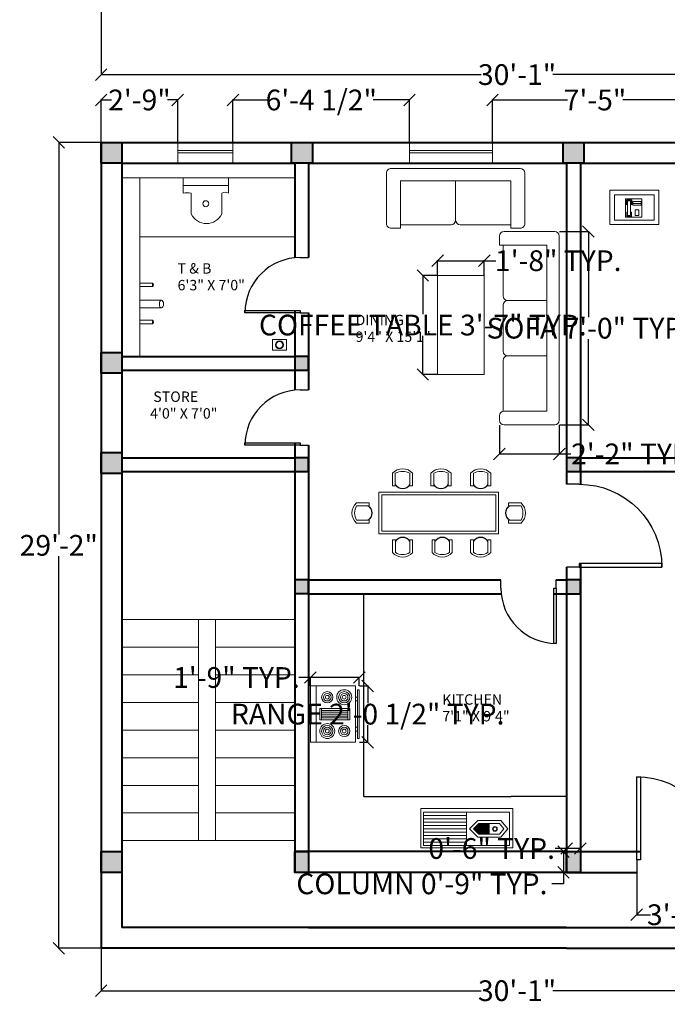
# Model space of a CAD drawing. Units: inches. Extents: x -19 to 1000, y -122 to 1144.
# Tile 4 of 8: x 529 to 810, y -115 to 313. Entities that reach past the tile are written whole.
import ezdxf

# ---------------------------------------------------------------- set-up
doc = ezdxf.new("R2010")
doc.units = ezdxf.units.IN
doc.header["$MEASUREMENT"] = 0
for name, color, linetype, lineweight in [('A-ANNO-DIMS', 191, 'Continuous', 18), ('A-AREA-IDEN', 1, 'Continuous', 18), ('A-COLS', 4, 'Continuous', 40), ('A-COLS-PATT', 220, 'Continuous', 13), ('A-EQPM', 120, 'Continuous', 18), ('A-FLOR-CASE', 254, 'Continuous', 25), ('A-FLOR-FIXT', 8, 'Continuous', 18), ('A-FLOR-STRS', 241, 'Continuous', 18), ('DOORS', 2, 'Continuous', 25), ('FURNITURE', 120, 'Continuous', 18), ('WALLS', 4, 'Continuous', 40), ('WINDOWS', 3, 'Continuous', 18)]:
    doc.layers.add(name, color=color, linetype=linetype, lineweight=lineweight)
doc.styles.get("Standard").update_dxf_attribs({"font": 'arial.ttf'})
doc.dimstyles.get("Standard").update_dxf_attribs({"dimtxt": 9, "dimasz": 5, "dimexe": 0.18, "dimexo": 0.0625, "dimgap": 0.09, "dimtad": 0, "dimtih": 1, "dimtoh": 1, "dimdec": 0, "dimzin": 0, "dimdsep": 46, "dimlunit": 3, "dimtxsty": 'Standard', "dimblk": 'OBLIQUE', "dimcen": 0.09, "dimadec": 0, "dimazin": 0, "dimtfac": 1, "dimtdec": 0, "dimtofl": 0, "dimtmove": 0, "dimatfit": 3, "dimfxl": 1, "dimtolj": 1, "dimtzin": 0, "dimarcsym": 0})

# ---------------------------------------------------------------- blocks, each defined once
blk = doc.blocks.new('Phone - Desk')
for p, q in [((-4.5, -5), (-4.5, 5)), ((-4.5, 5), (4.5, 5)), ((-4, 4.5), (-4, 2)), ((-4, 2), (-3.25, 2)), ((-3.75, 4.5), (-3.75, 2.25)), ((-1.25, 4.5), (-3.75, 4.5)), ((-3.75, 2.25), (-3.25, 2.25)), ((-3.25, 4), (-3.25, -4)), ((-3.25, 4), (-1.75, 4)), ((-1.75, -4), (-1.75, 4)), ((-1.75, 2.25), (-1.25, 2.25)), ((-1.75, 2), (-1, 2)), ((-1.25, 2.25), (-1.25, 4.5)), ((-1, 2), (-1, 4.5)), ((4, 3.5), (-0.5, 3.5)), ((-0.5, 3.5), (-0.5, 1.5)), ((-0.5, 2.5), (4, 2.5)), ((-0.5, 1.5), (4, 1.5)), ((4, 1.5), (4, 3.5)), ((4.5, 5), (4.5, -5)), ((4.5, -5), (-4.5, -5)), ((-3.75, -2.25), (-3.25, -2.25)), ((-3.75, -4.5), (-3.75, -2.25)), ((-1.25, -4.5), (-3.75, -4.5)), ((-3.25, -4), (-1.75, -4)), ((-1.75, -2.25), (-1.25, -2.25)), ((-1.25, -2.25), (-1.25, -4.5)), ((2.75, -1), (0.75, -1)), ((0.75, -1), (0.75, -4)), ((0.75, -4), (2.75, -4)), ((2.75, -4), (2.75, -1))]:
    blk.add_line(p, q)
blk = doc.blocks.new('Range-Oven - 30 in top')
for p, q in [((0, -3), (30, -3)), ((12, -6), (18, -6)), ((13, -20), (13, -6)), ((14, -6), (14, -20)), ((15, -20), (15, -6)), ((16, -6), (16, -20)), ((17, -20), (17, -6)), ((18, -20), (12, -20)), ((6, -24), (6, -25)), ((8, -25), (8, -24)), ((22, -25), (22, -24)), ((24, -24), (24, -25))]:
    blk.add_line(p, q)
for points in [[(0, -24), (0, 0), (30, 0), (30, -24)], [(12, -21), (12, -5), (18, -5), (18, -21)], [(2, -26), (2, -25), (28, -25), (28, -26)]]:
    blk.add_lwpolyline(points, close=True)
for centre, radius in [((6, -9), 4), ((6, -9), 3), ((6, -9), 2), ((6, -9), 1), ((24, -9), 3), ((24, -9), 2), ((24, -9), 1), ((6, -18), 3), ((24, -18), 4), ((24, -18), 3), ((6, -18), 2), ((6, -18), 1), ((24, -18), 2), ((24, -18), 1)]:
    blk.add_circle(centre, radius)
blk = doc.blocks.new('*U3')
for p, q in [((0, 0), (0, -6)), ((40, 0), (40, -6))]:
    blk.add_line(p, q)
blk.add_lwpolyline([(0, 0), (0, 40), (1.75, 40), (1.75, 0)], close=True)
blk.add_arc((0, 0), 40, 0, 90)
blk = doc.blocks.new('SOFA-THREE-SEAT')
for p, q in [((0, 78), (0, 82)), ((2, 84), (24, 84)), ((26, 82), (26, 2)), ((0, 78), (20.62, 78)), ((1.56, 78), (1.56, 56)), ((20.62, 78), (20.62, 6)), ((1.56, 52), (1.56, 32)), ((3.56, 54), (20.62, 54)), ((3.56, 54), (3.56, 54)), ((3.56, 30), (20.62, 30)), ((3.56, 30), (3.56, 30)), ((1.56, 28), (1.56, 6)), ((2, 6), (20.62, 6)), ((0, 2), (0, 4)), ((24, 0), (2, 0))]:
    blk.add_line(p, q)
for centre, start, end in [((2, 82), 90, 180), ((24, 82), 0, 90), ((3.56, 56), 180, 270), ((3.56, 52), 90, 180), ((3.56, 32), 180, 270), ((3.56, 28), 90, 180), ((2, 4), 90, 180), ((2, 2), 180, 270), ((24, 2), 270, 0)]:
    blk.add_arc(centre, 2, start, end)
blk = doc.blocks.new('LOVESEAT')
for p, q in [((6, 20.62), (54, 20.62)), ((6, 0), (6, 20.62)), ((30, 3.56), (30, 20.62)), ((54, 0), (54, 20.62)), ((6, 1.56), (28, 1.56)), ((30, 3.56), (30, 3.56)), ((32, 1.56), (54, 1.56))]:
    blk.add_line(p, q)
blk.add_lwpolyline([(6, 0), (2, 0, -0.414214), (0, 2), (0, 24, -0.414214), (2, 26), (58, 26, -0.414213), (60, 24), (60, 2, -0.414214), (58, 0), (54, 0)], format="xyb")
for centre, start, end in [((28, 3.56), 270, 0), ((32, 3.56), 180, 270)]:
    blk.add_arc(centre, 2, start, end)
blk = doc.blocks.new('TABLE-COFFEE')
blk.add_lwpolyline([(20.25, 0), (0, 0), (0, 43), (20.25, 43)], close=True)
blk = doc.blocks.new('TABLE-DINING')
for points in [[(51.97, 0), (0, 0), (0, 18.2), (51.97, 18.2)], [(50.72, 1.24), (1.24, 1.24), (1.24, 16.96), (50.72, 16.96)]]:
    blk.add_lwpolyline(points, close=True)
blk = doc.blocks.new('TABLE-BEDSIDE')
for points in [[(0, 0), (21.2, 0), (21.2, 14.94), (0, 14.94)], [(2, 2), (19.2, 2), (19.2, 12.94), (2, 12.94)]]:
    blk.add_lwpolyline(points, close=True)
blk = doc.blocks.new('CHAIR-DINING')
for p, q in [((0, 1.28), (0, 6.78)), ((1.24, 1.28), (1.24, 6.78)), ((7.52, 1.28), (7.52, 6.78)), ((8.77, 1.28), (8.77, 6.78)), ((0, 1.28), (1.24, 1.28)), ((7.52, 1.28), (8.77, 1.28))]:
    blk.add_line(p, q)
for centre, radius, start, end in [((4.38, 2.88), 5.87, 41.6504, 138.3496), ((4.38, 1.47), 6.17, 59.4137, 120.5863), ((4.38, 3.81), 3.65, 210.7965, 329.2035), ((4.38, 3.65), 3.65, 210.7965, 329.2035)]:
    blk.add_arc(centre, radius, start, end)
blk = doc.blocks.new('SINK-WITH-DRAINBOARD')
for p, q in [((19.91, 15.5), (1.26, 15.5)), ((19.91, 14.06), (1.26, 14.06)), ((19.91, 1.08), (19.91, 15.5)), ((19.91, 12.62), (1.26, 12.62)), ((19.91, 11.17), (1.26, 11.17)), ((19.91, 9.73), (1.26, 9.73)), ((24.75, 11.88), (21.21, 8.28)), ((25.28, 10.62), (22.97, 8.28)), ((23.36, 8.67), (29.71, 8.67)), ((23.74, 9.06), (29.71, 9.06)), ((24.12, 9.45), (29.71, 9.45)), ((24.51, 9.84), (29.71, 9.84)), ((24.75, 11.88), (34.73, 11.88)), ((24.89, 10.23), (29.71, 10.23)), ((25.28, 10.62), (34.14, 10.62)), ((25.28, 10.62), (29.71, 10.62)), ((29.71, 5.94), (29.71, 10.62)), ((34.14, 10.62), (36.12, 8.28)), ((34.73, 11.88), (37.76, 8.28)), ((19.91, 8.29), (1.26, 8.29)), ((19.91, 6.85), (1.26, 6.85)), ((19.91, 5.4), (1.26, 5.4)), ((24.75, 4.68), (21.21, 8.28)), ((25.28, 5.94), (22.97, 8.28)), ((22.97, 8.28), (29.71, 8.28)), ((23.36, 7.89), (29.71, 7.89)), ((23.74, 7.5), (29.71, 7.5)), ((24.12, 7.11), (29.71, 7.11)), ((24.51, 6.72), (29.71, 6.72)), ((24.75, 4.68), (34.73, 4.68)), ((24.89, 6.33), (29.71, 6.33)), ((25.28, 5.94), (34.14, 5.94)), ((34.14, 5.94), (36.12, 8.28)), ((34.73, 4.68), (37.76, 8.28)), ((19.91, 3.96), (1.26, 3.96)), ((19.91, 2.52), (1.26, 2.52))]:
    blk.add_line(p, q)
for points in [[(40, 0), (0, 0), (0, 17.1), (40, 17.1)], [(38.55, 1.08), (1.26, 1.08), (1.26, 15.5), (38.55, 15.5)]]:
    blk.add_lwpolyline(points, close=True)
for radius in [1.01, 0.803]:
    blk.add_circle((32.21, 8.28), radius)
blk = doc.blocks.new('WC-PLAN')
for p, q in [((0, 13.24), (0, 19.84)), ((0, 19.84), (19.57, 19.84)), ((19.57, 13.24), (19.57, 19.84)), ((0, 16.54), (19.57, 16.54)), ((3.44, 13.24), (3.44, 4.14)), ((16.7, 13.24), (16.7, 4.14))]:
    blk.add_line(p, q)
blk.add_circle((9.78, 8.6), 1.3)
for centre, radius, start, end in [((1.72, 2.24), 11.13, 81.1156, 98.8844), ((18.13, 10.18), 3.38, 64.9191, 115.0809), ((10.07, 7.39), 7.39, 206.0978, 333.9022)]:
    blk.add_arc(centre, radius, start, end)
blk = doc.blocks.new('FLOOR-DRAIN')
blk.add_lwpolyline([(6.19, 0), (0, 0), (0, 4.58), (6.19, 4.58)], close=True)
for radius in [1.73, 1.73, 1.73, 1.49]:
    blk.add_circle((3.09, 2.29), radius)
blk = doc.blocks.new('STAIR-RETURN-PLAN')
for p, q in [((75, 96), (0, 96)), ((33.21, 0), (33.21, 96)), ((40.68, 0), (40.68, 96)), ((33.21, 84), (0, 84)), ((75, 84), (40.68, 84)), ((33.21, 72), (0, 72)), ((75, 72), (40.68, 72)), ((33.21, 60), (0, 60)), ((75, 60), (40.68, 60)), ((33.21, 48), (0, 48)), ((75, 48), (40.68, 48)), ((33.21, 36), (0, 36)), ((75, 36), (40.68, 36)), ((33.21, 24), (0, 24)), ((75, 24), (40.68, 24)), ((33.21, 12), (0, 12)), ((75, 12), (40.68, 12)), ((75, 0), (0, 0))]:
    blk.add_line(p, q)
blk = doc.blocks.new('WIN-24-PLAN')
for p, q in [((0, 4.5), (0, 9)), ((0, 9), (0, 0)), ((24, 9), (24, 0)), ((0, 5.5), (24, 5.5)), ((0, 4.5), (24, 4.5))]:
    blk.add_line(p, q)
blk = doc.blocks.new('WIN-36-PLAN')
for p, q in [((0, 4.5), (0, 9)), ((0, 9), (0, 0)), ((36, 9), (36, 0)), ((0, 5.5), (36, 5.5)), ((0, 5.5), (36, 5.5)), ((0, 4.5), (36, 4.5))]:
    blk.add_line(p, q)
blk = doc.blocks.new('COLUMN-9X9')
blk.add_lwpolyline([(0, 9), (9, 9), (9, 0), (0, 0)], close=True)
blk = doc.blocks.new('COLUMN-6X6')
blk.add_lwpolyline([(6, 6), (0, 6), (0, 0), (6, 0)], close=True)
blk = doc.blocks.new('COLUMN-6X9')
blk.add_lwpolyline([(0, 9), (6, 9), (6, 0), (0, 0)], close=True)
blk = doc.blocks.new('_Oblique')
at = {"color": 0, "linetype": 'ByBlock', "lineweight": -2}
blk.add_line((-0.5, -0.5), (0.5, 0.5), dxfattribs=at)
blk = doc.blocks.new('*D37')
at = {"layer": 'A-ANNO-DIMS', "color": 0, "lineweight": -2, "transparency": 16777216}
for p, q in [((766.28, -48.29), (764.81, -48.29)), ((764.99, -48.29), (764.99, -57.29)), ((766.28, -57.29), (764.81, -57.29)), ((764.99, -57.29), (764.99, -62.29)), ((764.99, -62.29), (759.99, -62.29))]:
    blk.add_line(p, q, dxfattribs=at)
at = {"layer": 'Defpoints', "color": 0, "transparency": 16777216}
for p in [(766.34, -48.29), (764.99, -57.29), (766.34, -57.29)]:
    blk.add_point(p, dxfattribs=at)
at = {"layer": 'A-ANNO-DIMS', "color": 0, "lineweight": -2, "transparency": 16777216, "xscale": 5, "yscale": 5, "zscale": 5}
for p, rotation in [((764.99, -48.29), 90), ((764.99, -57.29), 270)]:
    blk.add_blockref('_Oblique', p, dxfattribs=dict(at, rotation=rotation))
at = {"layer": 'A-ANNO-DIMS', "color": 0, "transparency": 16777216, "insert": (703.54, -62.29), "char_height": 9, "attachment_point": 5}
blk.add_mtext('\\A1;COLUMN 0\'-9" TYP.', dxfattribs=at)
blk = doc.blocks.new('*D38')
at = {"layer": 'A-ANNO-DIMS', "color": 0, "lineweight": -2, "transparency": 16777216}
for p, q in [((766.34, -46.94), (761.34, -46.94)), ((766.34, -48.23), (766.34, -46.76)), ((772.34, -46.94), (766.34, -46.94)), ((772.34, -48.23), (772.34, -46.76))]:
    blk.add_line(p, q, dxfattribs=at)
at = {"layer": 'Defpoints', "color": 0, "transparency": 16777216}
for p in [(766.34, -46.94), (766.34, -48.29), (772.34, -48.29)]:
    blk.add_point(p, dxfattribs=at)
at = {"layer": 'A-ANNO-DIMS', "color": 0, "lineweight": -2, "transparency": 16777216, "xscale": 5, "yscale": 5, "zscale": 5, "rotation": 180}
blk.add_blockref('_Oblique', (766.34, -46.94), dxfattribs=at)
at = {"layer": 'A-ANNO-DIMS', "color": 0, "lineweight": -2, "transparency": 16777216, "xscale": 5, "yscale": 5, "zscale": 5}
blk.add_blockref('_Oblique', (772.34, -46.94), dxfattribs=at)
at = {"layer": 'A-ANNO-DIMS', "color": 0, "transparency": 16777216, "insert": (733.82, -46.94), "char_height": 9, "attachment_point": 5}
blk.add_mtext('\\A1;0\'-6" TYP.', dxfattribs=at)
blk = doc.blocks.new('*D51')
at = {"layer": 'A-ANNO-DIMS', "color": 0, "lineweight": -2, "transparency": 16777216}
for p, q in [((676.41, 23.65), (680.2, 23.65)), ((680.02, 23.65), (680.02, 16.16)), ((680.02, -0.82), (680.02, 6.67)), ((676.41, -0.82), (680.2, -0.82))]:
    blk.add_line(p, q, dxfattribs=at)
at = {"layer": 'Defpoints', "color": 0, "transparency": 16777216}
for p in [(676.35, 23.65), (680.02, 23.65), (676.35, -0.82)]:
    blk.add_point(p, dxfattribs=at)
at = {"layer": 'A-ANNO-DIMS', "color": 0, "lineweight": -2, "transparency": 16777216, "xscale": 5, "yscale": 5, "zscale": 5}
for p, rotation in [((680.02, 23.65), 90), ((680.02, -0.82), 270)]:
    blk.add_blockref('_Oblique', p, dxfattribs=dict(at, rotation=rotation))
at = {"layer": 'A-ANNO-DIMS', "color": 0, "transparency": 16777216, "insert": (680.02, 11.41), "char_height": 9, "attachment_point": 5}
blk.add_mtext('\\A1;RANGE 2\'-0 1/2" TYP.', dxfattribs=at)
blk = doc.blocks.new('*D52')
at = {"layer": 'A-ANNO-DIMS', "color": 0, "lineweight": -2, "transparency": 16777216}
for p, q in [((655.14, 27.32), (650.14, 27.32)), ((655.14, 23.71), (655.14, 27.5)), ((676.35, 27.32), (655.14, 27.32)), ((676.35, 23.71), (676.35, 27.5))]:
    blk.add_line(p, q, dxfattribs=at)
at = {"layer": 'Defpoints', "color": 0, "transparency": 16777216}
for p in [(655.14, 27.32), (655.14, 23.65), (676.35, 23.65)]:
    blk.add_point(p, dxfattribs=at)
at = {"layer": 'A-ANNO-DIMS', "color": 0, "lineweight": -2, "transparency": 16777216, "xscale": 5, "yscale": 5, "zscale": 5, "rotation": 180}
blk.add_blockref('_Oblique', (655.14, 27.32), dxfattribs=at)
at = {"layer": 'A-ANNO-DIMS', "color": 0, "lineweight": -2, "transparency": 16777216, "xscale": 5, "yscale": 5, "zscale": 5}
blk.add_blockref('_Oblique', (676.35, 27.32), dxfattribs=at)
at = {"layer": 'A-ANNO-DIMS', "color": 0, "transparency": 16777216, "insert": (623.05, 27.32), "char_height": 9, "attachment_point": 5}
blk.add_mtext('\\A1;1\'-9" TYP.', dxfattribs=at)
blk = doc.blocks.new('*D53')
at = {"layer": 'A-ANNO-DIMS', "color": 0, "lineweight": -2, "transparency": 16777216}
for p, q in [((763.25, 221.01), (775.96, 221.01)), ((775.78, 221.01), (775.78, 183.75)), ((775.78, 137.01), (775.78, 174.26)), ((763.25, 137.01), (775.96, 137.01))]:
    blk.add_line(p, q, dxfattribs=at)
at = {"layer": 'Defpoints', "color": 0, "transparency": 16777216}
for p in [(763.18, 221.01), (775.78, 221.01), (763.18, 137.01)]:
    blk.add_point(p, dxfattribs=at)
at = {"layer": 'A-ANNO-DIMS', "color": 0, "lineweight": -2, "transparency": 16777216, "xscale": 5, "yscale": 5, "zscale": 5}
for p, rotation in [((775.78, 221.01), 90), ((775.78, 137.01), 270)]:
    blk.add_blockref('_Oblique', p, dxfattribs=dict(at, rotation=rotation))
at = {"layer": 'A-ANNO-DIMS', "color": 0, "transparency": 16777216, "insert": (775.78, 179.01), "char_height": 9, "attachment_point": 5}
blk.add_mtext('\\A1;SOFA 7\'-0" TYP.', dxfattribs=at)
blk = doc.blocks.new('*D54')
at = {"layer": 'A-ANNO-DIMS', "color": 0, "lineweight": -2, "transparency": 16777216}
for p, q in [((737.18, 136.94), (737.18, 124.23)), ((763.18, 136.94), (763.18, 124.23)), ((737.18, 124.41), (763.18, 124.41)), ((763.18, 124.41), (768.18, 124.41))]:
    blk.add_line(p, q, dxfattribs=at)
at = {"layer": 'Defpoints', "color": 0, "transparency": 16777216}
for p in [(737.18, 137.01), (763.18, 137.01), (763.18, 124.41)]:
    blk.add_point(p, dxfattribs=at)
at = {"layer": 'A-ANNO-DIMS', "color": 0, "lineweight": -2, "transparency": 16777216, "xscale": 5, "yscale": 5, "zscale": 5, "rotation": 180}
blk.add_blockref('_Oblique', (737.18, 124.41), dxfattribs=at)
at = {"layer": 'A-ANNO-DIMS', "color": 0, "lineweight": -2, "transparency": 16777216, "xscale": 5, "yscale": 5, "zscale": 5}
blk.add_blockref('_Oblique', (763.18, 124.41), dxfattribs=at)
at = {"layer": 'A-ANNO-DIMS', "color": 0, "transparency": 16777216, "insert": (795.78, 124.41), "char_height": 9, "attachment_point": 5}
blk.add_mtext('\\A1;2\'-2" TYP.', dxfattribs=at)
blk = doc.blocks.new('*D57')
at = {"layer": 'A-ANNO-DIMS', "color": 0, "lineweight": -2, "transparency": 16777216}
for p, q in [((710.31, 201.87), (703.74, 201.87)), ((703.92, 201.87), (703.92, 185.12)), ((703.92, 158.87), (703.92, 175.62)), ((710.31, 158.87), (703.74, 158.87))]:
    blk.add_line(p, q, dxfattribs=at)
at = {"layer": 'Defpoints', "color": 0, "transparency": 16777216}
for p in [(703.92, 201.87), (710.37, 201.87), (710.37, 158.87)]:
    blk.add_point(p, dxfattribs=at)
at = {"layer": 'A-ANNO-DIMS', "color": 0, "lineweight": -2, "transparency": 16777216, "xscale": 5, "yscale": 5, "zscale": 5}
for p, rotation in [((703.92, 201.87), 90), ((703.92, 158.87), 270)]:
    blk.add_blockref('_Oblique', p, dxfattribs=dict(at, rotation=rotation))
at = {"layer": 'A-ANNO-DIMS', "color": 0, "transparency": 16777216, "insert": (703.92, 180.37), "char_height": 9, "attachment_point": 5}
blk.add_mtext('\\A1;COFFEE TABLE 3\'-7" TYP.', dxfattribs=at)
blk = doc.blocks.new('*D58')
at = {"layer": 'A-ANNO-DIMS', "color": 0, "lineweight": -2, "transparency": 16777216}
for p, q in [((710.37, 201.93), (710.37, 208.5)), ((710.37, 208.32), (730.62, 208.32)), ((730.62, 201.93), (730.62, 208.5)), ((730.62, 208.32), (735.62, 208.32))]:
    blk.add_line(p, q, dxfattribs=at)
at = {"layer": 'Defpoints', "color": 0, "transparency": 16777216}
for p in [(730.62, 208.32), (710.37, 201.87), (730.62, 201.87)]:
    blk.add_point(p, dxfattribs=at)
at = {"layer": 'A-ANNO-DIMS', "color": 0, "lineweight": -2, "transparency": 16777216, "xscale": 5, "yscale": 5, "zscale": 5, "rotation": 180}
blk.add_blockref('_Oblique', (710.37, 208.32), dxfattribs=at)
at = {"layer": 'A-ANNO-DIMS', "color": 0, "lineweight": -2, "transparency": 16777216, "xscale": 5, "yscale": 5, "zscale": 5}
blk.add_blockref('_Oblique', (730.62, 208.32), dxfattribs=at)
at = {"layer": 'A-ANNO-DIMS', "color": 0, "transparency": 16777216, "insert": (762.72, 208.32), "char_height": 9, "attachment_point": 5}
blk.add_mtext('\\A1;1\'-8" TYP.', dxfattribs=at)
blk = doc.blocks.new('*D103')
at = {"layer": 'A-ANNO-DIMS', "color": 0, "lineweight": -2, "transparency": 16777216}
for p, q in [((564.34, -90.36), (564.34, -108.87)), ((925.34, -90.36), (925.34, -108.87)), ((564.34, -108.69), (729.3, -108.69)), ((925.34, -108.69), (760.39, -108.69))]:
    blk.add_line(p, q, dxfattribs=at)
at = {"layer": 'Defpoints', "color": 0, "transparency": 16777216}
for p in [(564.34, -90.29), (925.34, -90.29), (925.34, -108.69)]:
    blk.add_point(p, dxfattribs=at)
at = {"layer": 'A-ANNO-DIMS', "color": 0, "lineweight": -2, "transparency": 16777216, "xscale": 5, "yscale": 5, "zscale": 5, "rotation": 180}
blk.add_blockref('_Oblique', (564.34, -108.69), dxfattribs=at)
at = {"layer": 'A-ANNO-DIMS', "color": 0, "lineweight": -2, "transparency": 16777216, "xscale": 5, "yscale": 5, "zscale": 5}
blk.add_blockref('_Oblique', (925.34, -108.69), dxfattribs=at)
at = {"layer": 'A-ANNO-DIMS', "color": 0, "transparency": 16777216, "insert": (744.84, -108.69), "char_height": 9, "attachment_point": 5}
blk.add_mtext('\\A1;30\'-1"', dxfattribs=at)
blk = doc.blocks.new('*D104')
at = {"layer": 'A-ANNO-DIMS', "color": 0, "lineweight": -2, "transparency": 16777216}
for p, q in [((564.28, 259.71), (545.76, 259.71)), ((545.94, 259.71), (545.94, 89.39)), ((545.94, -90.29), (545.94, 80.02)), ((564.28, -90.29), (545.76, -90.29))]:
    blk.add_line(p, q, dxfattribs=at)
at = {"layer": 'Defpoints', "color": 0, "transparency": 16777216}
for p in [(545.94, 259.71), (564.34, 259.71), (564.34, -90.29)]:
    blk.add_point(p, dxfattribs=at)
at = {"layer": 'A-ANNO-DIMS', "color": 0, "lineweight": -2, "transparency": 16777216, "xscale": 5, "yscale": 5, "zscale": 5}
for p, rotation in [((545.94, 259.71), 90), ((545.94, -90.29), 270)]:
    blk.add_blockref('_Oblique', p, dxfattribs=dict(at, rotation=rotation))
at = {"layer": 'A-ANNO-DIMS', "color": 0, "transparency": 16777216, "insert": (545.94, 84.71), "char_height": 9, "attachment_point": 5}
blk.add_mtext('\\A1;29\'-2"', dxfattribs=at)
blk = doc.blocks.new('*D105')
at = {"layer": 'A-ANNO-DIMS', "color": 0, "lineweight": -2, "transparency": 16777216}
for p, q in [((564.34, 259.77), (564.34, 278.29)), ((564.34, 278.11), (568.82, 278.11)), ((597.55, 278.11), (593.08, 278.11)), ((597.55, 259.77), (597.55, 278.29))]:
    blk.add_line(p, q, dxfattribs=at)
at = {"layer": 'Defpoints', "color": 0, "transparency": 16777216}
for p in [(597.55, 278.11), (564.34, 259.71), (597.55, 259.71)]:
    blk.add_point(p, dxfattribs=at)
at = {"layer": 'A-ANNO-DIMS', "color": 0, "lineweight": -2, "transparency": 16777216, "xscale": 5, "yscale": 5, "zscale": 5, "rotation": 180}
blk.add_blockref('_Oblique', (564.34, 278.11), dxfattribs=at)
at = {"layer": 'A-ANNO-DIMS', "color": 0, "lineweight": -2, "transparency": 16777216, "xscale": 5, "yscale": 5, "zscale": 5}
blk.add_blockref('_Oblique', (597.55, 278.11), dxfattribs=at)
at = {"layer": 'A-ANNO-DIMS', "color": 0, "transparency": 16777216, "insert": (580.95, 278.11), "char_height": 9, "attachment_point": 5}
blk.add_mtext('\\A1;2\'-9"', dxfattribs=at)
blk = doc.blocks.new('*D106')
at = {"layer": 'A-ANNO-DIMS', "color": 0, "lineweight": -2, "transparency": 16777216}
for p, q in [((621.55, 259.77), (621.55, 278.29)), ((621.55, 278.11), (637.3, 278.11)), ((698.18, 278.11), (682.43, 278.11)), ((698.18, 259.77), (698.18, 278.29))]:
    blk.add_line(p, q, dxfattribs=at)
at = {"layer": 'Defpoints', "color": 0, "transparency": 16777216}
for p in [(698.18, 278.11), (621.55, 259.71), (698.18, 259.71)]:
    blk.add_point(p, dxfattribs=at)
at = {"layer": 'A-ANNO-DIMS', "color": 0, "lineweight": -2, "transparency": 16777216, "xscale": 5, "yscale": 5, "zscale": 5, "rotation": 180}
blk.add_blockref('_Oblique', (621.55, 278.11), dxfattribs=at)
at = {"layer": 'A-ANNO-DIMS', "color": 0, "lineweight": -2, "transparency": 16777216, "xscale": 5, "yscale": 5, "zscale": 5}
blk.add_blockref('_Oblique', (698.18, 278.11), dxfattribs=at)
at = {"layer": 'A-ANNO-DIMS', "color": 0, "transparency": 16777216, "insert": (659.87, 278.11), "char_height": 9, "attachment_point": 5}
blk.add_mtext('\\A1;6\'-4 1/2"', dxfattribs=at)
blk = doc.blocks.new('*D107')
at = {"layer": 'A-ANNO-DIMS', "color": 0, "lineweight": -2, "transparency": 16777216}
for p, q in [((734.18, 259.77), (734.18, 278.29)), ((734.18, 278.11), (766.67, 278.11)), ((823.18, 278.11), (790.7, 278.11)), ((823.18, 259.77), (823.18, 278.29))]:
    blk.add_line(p, q, dxfattribs=at)
at = {"layer": 'Defpoints', "color": 0, "transparency": 16777216}
for p in [(823.18, 278.11), (734.18, 259.71), (823.18, 259.71)]:
    blk.add_point(p, dxfattribs=at)
at = {"layer": 'A-ANNO-DIMS', "color": 0, "lineweight": -2, "transparency": 16777216, "xscale": 5, "yscale": 5, "zscale": 5, "rotation": 180}
blk.add_blockref('_Oblique', (734.18, 278.11), dxfattribs=at)
at = {"layer": 'A-ANNO-DIMS', "color": 0, "lineweight": -2, "transparency": 16777216, "xscale": 5, "yscale": 5, "zscale": 5}
blk.add_blockref('_Oblique', (823.18, 278.11), dxfattribs=at)
at = {"layer": 'A-ANNO-DIMS', "color": 0, "transparency": 16777216, "insert": (778.68, 278.11), "char_height": 9, "attachment_point": 5}
blk.add_mtext('\\A1;7\'-5"', dxfattribs=at)
blk = doc.blocks.new('*D109')
at = {"layer": 'A-ANNO-DIMS', "color": 0, "lineweight": -2, "transparency": 16777216}
for p, q in [((796.78, -57.36), (796.78, -75.87)), ((832.78, -57.36), (832.78, -75.87)), ((796.78, -75.69), (802.73, -75.69)), ((832.78, -75.69), (826.83, -75.69))]:
    blk.add_line(p, q, dxfattribs=at)
at = {"layer": 'Defpoints', "color": 0, "transparency": 16777216}
for p in [(796.78, -57.29), (832.78, -57.29), (796.78, -75.69)]:
    blk.add_point(p, dxfattribs=at)
at = {"layer": 'A-ANNO-DIMS', "color": 0, "lineweight": -2, "transparency": 16777216, "xscale": 5, "yscale": 5, "zscale": 5, "rotation": 180}
blk.add_blockref('_Oblique', (796.78, -75.69), dxfattribs=at)
at = {"layer": 'A-ANNO-DIMS', "color": 0, "lineweight": -2, "transparency": 16777216, "xscale": 5, "yscale": 5, "zscale": 5}
blk.add_blockref('_Oblique', (832.78, -75.69), dxfattribs=at)
at = {"layer": 'A-ANNO-DIMS', "color": 0, "transparency": 16777216, "insert": (814.78, -75.69), "char_height": 9, "attachment_point": 5}
blk.add_mtext('\\A1;3\'-0"', dxfattribs=at)
blk = doc.blocks.new('*D129')
at = {"layer": 'A-ANNO-DIMS', "color": 0, "lineweight": -2, "transparency": 16777216}
for p, q in [((564.34, 328.07), (564.34, 288.95)), ((925.34, 328.07), (925.34, 288.95)), ((564.34, 289.13), (729.3, 289.13)), ((925.34, 289.13), (760.39, 289.13))]:
    blk.add_line(p, q, dxfattribs=at)
at = {"layer": 'Defpoints', "color": 0, "transparency": 16777216}
for p in [(564.34, 328.13), (925.34, 328.13), (925.34, 289.13)]:
    blk.add_point(p, dxfattribs=at)
at = {"layer": 'A-ANNO-DIMS', "color": 0, "lineweight": -2, "transparency": 16777216, "xscale": 5, "yscale": 5, "zscale": 5, "rotation": 180}
blk.add_blockref('_Oblique', (564.34, 289.13), dxfattribs=at)
at = {"layer": 'A-ANNO-DIMS', "color": 0, "lineweight": -2, "transparency": 16777216, "xscale": 5, "yscale": 5, "zscale": 5}
blk.add_blockref('_Oblique', (925.34, 289.13), dxfattribs=at)
at = {"layer": 'A-ANNO-DIMS', "color": 0, "transparency": 16777216, "insert": (744.84, 289.13), "char_height": 9, "attachment_point": 5}
blk.add_mtext('\\A1;30\'-1"', dxfattribs=at)

msp = doc.modelspace()

# ---------------------------------------------------------------- hatches: boundary and pattern name
at = {"layer": 'A-COLS-PATT'}
h = msp.add_hatch(color=256, dxfattribs=at)
h.dxf.hatch_style = 1
h.paths.add_polyline_path([(573.34, 259.71), (564.34, 259.71), (564.34, 250.71), (573.34, 250.71)])
h.paths.add_polyline_path([(656.01, 259.71), (647.01, 259.71), (647.01, 250.71), (656.01, 250.71)])
h.paths.add_polyline_path([(773.81, 259.71), (764.81, 259.71), (764.81, 250.71), (773.81, 250.71)])
h.paths.add_polyline_path([(925.34, 259.71), (916.34, 259.71), (916.34, 250.71), (925.34, 250.71)])
h = msp.add_hatch(color=256, dxfattribs=at)
h.dxf.hatch_style = 1
h.paths.add_polyline_path([(573.34, 168.48), (564.34, 168.48), (564.34, 159.48), (573.34, 159.48)])
h.paths.add_polyline_path([(654.34, 166.71), (648.34, 166.71), (648.34, 160.71), (654.34, 160.71)])
h.paths.add_polyline_path([(573.34, 124.97), (564.34, 124.97), (564.34, 115.97), (573.34, 115.97)])
h.paths.add_polyline_path([(654.34, 122.71), (648.34, 122.71), (648.34, 116.71), (654.34, 116.71)])
h.paths.add_polyline_path([(654.34, 69.8), (648.34, 69.8), (648.34, 63.8), (654.34, 63.8)])
h.paths.add_polyline_path([(772.34, 69.71), (766.34, 69.71), (766.34, 63.71), (772.34, 63.71)])
h.paths.add_polyline_path([(772.34, 122.71), (766.34, 122.71), (766.34, 116.71), (772.34, 116.71)])
h.paths.add_polyline_path([(925.34, 124.12), (916.34, 124.12), (916.34, 115.12), (925.34, 115.12)])
h.paths.add_polyline_path([(925.34, -48.29), (916.34, -48.29), (916.34, -57.29), (925.34, -57.29)])
h.paths.add_polyline_path([(772.34, -48.29), (766.34, -48.29), (766.34, -57.29), (772.34, -57.29)])
h.paths.add_polyline_path([(654.34, -48.29), (648.34, -48.29), (648.34, -57.29), (654.34, -57.29)])
h.paths.add_polyline_path([(573.34, -48.29), (564.34, -48.29), (564.34, -57.29), (573.34, -57.29)])

# ---------------------------------------------------------------- linework, layer by layer
at = {"layer": 'A-FLOR-CASE'}
for p, q in [((678.34, -24.29), (678.34, 63.71)), ((678.34, -24.29), (742.34, -24.29)), ((766.34, -24.29), (742.34, -24.29))]:
    msp.add_line(p, q, dxfattribs=at)
at = {"layer": 'A-FLOR-FIXT'}
for p, q in [((573.34, 244.3), (648.34, 244.3)), ((581.18, 166.71), (581.18, 244.3)), ((581.18, 218.69), (648.34, 218.69)), ((581.18, 198.59), (586.55, 198.59)), ((581.18, 197.08), (586.55, 197.08)), ((586.55, 198.59), (586.55, 197.08)), ((581.18, 191.12), (590.5, 191.12)), ((581.18, 187.85), (590.5, 187.85)), ((581.18, 182.45), (586.55, 182.45)), ((581.18, 180.94), (586.55, 180.94)), ((586.55, 182.45), (586.55, 180.94))]:
    msp.add_line(p, q, dxfattribs=at)
for centre in [(586.32, 197.83), (586.32, 181.69)]:
    msp.add_arc(centre, 0.786, 286.4895, 73.5105, dxfattribs=at)
msp.add_ellipse((590.5, 189.48), major_axis=(0, 1.63), ratio=0.555125, dxfattribs=at)
at = {"layer": 'WALLS'}
for p, q in [((564.34, 259.71), (564.34, -90.29)), ((564.34, 259.71), (925.34, 259.71)), ((573.34, 259.71), (573.34, -48.29)), ((573.34, 250.71), (648.34, 250.71)), ((648.34, 250.71), (648.34, 209.57)), ((654.34, 250.71), (654.34, 209.69)), ((654.34, 250.71), (766.34, 250.71)), ((766.34, 250.71), (766.34, 111.24)), ((772.34, 250.71), (772.34, 111.24)), ((772.34, 250.71), (916.34, 250.71)), ((648.34, 186.74), (648.34, 152.09)), ((654.34, 185.69), (654.34, 152.21)), ((573.34, 166.71), (648.34, 166.71)), ((573.34, 160.71), (648.34, 160.71)), ((648.34, 129.26), (648.34, -57.29)), ((654.34, 128.21), (654.34, -57.29)), ((573.34, 122.71), (648.34, 122.71)), ((772.34, 122.71), (916.34, 122.71)), ((573.34, 116.71), (648.34, 116.71)), ((772.34, 116.71), (916.34, 116.71)), ((766.34, 75.24), (766.34, -57.29)), ((772.34, 76.82), (772.34, -57.29)), ((654.34, 69.71), (737.83, 69.71)), ((761.83, 69.71), (766.34, 69.71)), ((654.34, 63.71), (737.95, 63.71)), ((760.78, 63.71), (766.34, 63.71)), ((766.34, -48.29), (648.34, -48.29)), ((766.34, -48.29), (798.35, -48.29)), ((573.34, -57.29), (573.34, -81.29)), ((766.34, -57.29), (648.34, -57.29)), ((766.34, -57.29), (796.78, -57.29)), ((766.34, -81.29), (573.34, -81.29)), ((654.34, -81.29), (916.34, -81.29)), ((766.34, -81.29), (654.34, -81.29)), ((654.34, -90.29), (564.34, -90.29)), ((766.34, -90.29), (654.34, -90.29)), ((766.34, -90.29), (925.34, -90.29))]:
    msp.add_line(p, q, dxfattribs=at)
msp.add_lwpolyline([(564.34, -57.29), (564.34, -48.29)], dxfattribs=at)

# ---------------------------------------------------------------- block references
at = {"layer": 'A-COLS'}
for p in [(564.34, 250.71), (647.01, 250.71), (764.81, 250.71), (564.34, 159.48), (564.34, 115.97), (564.34, -57.3)]:
    msp.add_blockref('COLUMN-9X9', p, dxfattribs=at)
for name, p, rotation in [('COLUMN-6X6', (648.34, 166.71), 270.0000000000003), ('COLUMN-6X6', (648.34, 122.71), 270.0000000000003), ('COLUMN-6X6', (766.34, 122.71), 270.0000000000013), ('COLUMN-6X6', (766.34, 122.71), 270.0000000000013), ('COLUMN-6X6', (648.34, 69.8), 270.0000000000003), ('COLUMN-6X6', (648.34, 69.8), 270.0000000000003), ('COLUMN-6X6', (766.34, 69.71), 270.0000000000013), ('COLUMN-6X9', (654.34, -48.29), 180), ('COLUMN-6X9', (772.34, -48.29), 180)]:
    msp.add_blockref(name, p, dxfattribs=dict(at, rotation=rotation))
at = {"layer": 'A-EQPM', "xscale": 0.8015722193121366, "yscale": 0.8015722193121366, "zscale": 0.8015722193121366}
msp.add_blockref('Phone - Desk', (795.45, 231.16), dxfattribs=at)
at = {"layer": 'A-EQPM', "xscale": 0.8155908971350484, "yscale": 0.8155908971350484, "zscale": 0.8155908971350484, "rotation": 90}
msp.add_blockref('Range-Oven - 30 in top', (655.14, -0.82), dxfattribs=at)
at = {"layer": 'A-FLOR-FIXT'}
for name, p in [('WC-PLAN', (599.97, 224.46)), ('FLOOR-DRAIN', (638.63, 169.51)), ('SINK-WITH-DRAINBOARD', (703.01, -46.69))]:
    msp.add_blockref(name, p, dxfattribs=at)
at = {"layer": 'A-FLOR-STRS'}
msp.add_blockref('STAIR-RETURN-PLAN', (573.34, -43.52), dxfattribs=at)
at = {"layer": 'DOORS'}
for p, xscale, yscale, zscale, rotation in [((650.74, 185.69), 0.6, 0.6, 0.6, 90), ((650.74, 128.21), 0.6, 0.6, 0.6, 90), ((771.74, 75.24), -0.9, 0.9, 0.9, 270), ((761.83, 66.11), 0.6, 0.6, 0.6, 180)]:
    msp.add_blockref('*U3', p, dxfattribs=dict(at, xscale=xscale, yscale=yscale, zscale=zscale, rotation=rotation))
at = {"layer": 'DOORS', "xscale": 0.9, "yscale": 0.9, "zscale": 0.9}
msp.add_blockref('*U3', (796.78, -51.89), dxfattribs=at)
at = {"layer": 'FURNITURE'}
for name, p in [('LOVESEAT', (688.19, 222.38)), ('TABLE-BEDSIDE', (785.15, 223.98)), ('SOFA-THREE-SEAT', (737.18, 137.01)), ('TABLE-COFFEE', (710.37, 158.87)), ('CHAIR-DINING', (690.76, 109.2)), ('CHAIR-DINING', (707.43, 109.2)), ('CHAIR-DINING', (724.65, 109.2)), ('TABLE-DINING', (684.88, 89.66))]:
    msp.add_blockref(name, p, dxfattribs=at)
for p, rotation in [((681.95, 94.37), 89.99999999999818), ((739.78, 103.14), 269.9999999999988), ((699.53, 88.32), 180), ((716.74, 88.32), 180), ((733.42, 88.32), 180)]:
    msp.add_blockref('CHAIR-DINING', p, dxfattribs=dict(at, rotation=rotation))
at = {"layer": 'WINDOWS'}
for name, p in [('WIN-24-PLAN', (597.55, 250.71)), ('WIN-36-PLAN', (698.18, 250.71))]:
    msp.add_blockref(name, p, dxfattribs=at)

# ---------------------------------------------------------------- texts
at = {"layer": 'A-AREA-IDEN'}
for s, height, p in [('T & B', 4.516, (597.49, 202.71)), ('6\'3" X 7\'0"', 4.5155, (597.49, 195.45)), ('DINING', 4.516, (674.75, 180.31)), ('9\'4" X 15\'1"', 4.5155, (674.75, 173.05)), (' STORE', 4.516, (585.57, 147.01)), ('4\'0" X 7\'0"', 4.5155, (585.57, 139.75)), ('KITCHEN', 4.516, (712.4, 15.51)), ('7\'1" X 9\'4"', 4.5155, (712.4, 8.25))]:
    msp.add_text(s, height=height, dxfattribs=at).set_placement(p)

# ---------------------------------------------------------------- dimensions: what is measured, and where the dimension line sits
at = {"layer": 'A-ANNO-DIMS'}
for base, p1, p2, picture, middle in [((925.34, 289.13), (564.34, 328.13), (925.34, 328.13), '*D129', (744.84, 289.13)), ((698.18, 278.11), (621.55, 259.71), (698.18, 259.71), '*D106', (659.87, 278.11)), ((597.55, 278.11), (564.34, 259.71), (597.55, 259.71), '*D105', (580.95, 278.11)), ((823.18, 278.11), (734.18, 259.71), (823.18, 259.71), '*D107', (778.68, 278.11)), ((925.34, -108.69), (564.34, -90.29), (925.34, -90.29), '*D103', (744.84, -108.69))]:
    dim = msp.add_linear_dim(base=base, p1=p1, p2=p2, dimstyle='Standard', override={"dimdec": 1, "dimlfac": 1, "dimrnd": 0, "dimzin": 1, "dimdsep": 46, "dimlunit": 4, "dimfrac": 2}, dxfattribs=at)
    dim.commit()
    dim.dimension.update_dxf_attribs({"geometry": picture, "text_midpoint": middle})
for base, p1, p2, angle, picture, middle in [((545.94, 259.71), (564.34, -90.29), (564.34, 259.71), 90, '*D104', (545.94, 84.71)), ((796.78, -75.69), (832.78, -57.29), (796.78, -57.29), 180, '*D109', (814.78, -75.69))]:
    dim = msp.add_linear_dim(base=base, p1=p1, p2=p2, angle=angle, dimstyle='Standard', override={"dimdec": 1, "dimlfac": 1, "dimrnd": 0, "dimzin": 1, "dimdsep": 46, "dimlunit": 4, "dimfrac": 2}, dxfattribs=at)
    dim.commit()
    dim.dimension.update_dxf_attribs({"geometry": picture, "text_midpoint": middle})
for base, p1, p2, angle, text, picture, middle in [((775.78, 221.01), (763.18, 137.01), (763.18, 221.01), 90, 'SOFA <> TYP.', '*D53', (775.78, 179.01)), ((703.92, 201.87), (710.37, 158.87), (710.37, 201.87), 90, 'COFFEE TABLE <> TYP.', '*D57', (703.92, 180.37)), ((655.14, 27.32), (676.35, 23.65), (655.14, 23.65), 180, '<> TYP.', '*D52', (623.05, 27.32)), ((680.02, 23.65), (676.35, -0.82), (676.35, 23.65), 90, 'RANGE <> TYP.', '*D51', (680.02, 11.41)), ((766.34, -46.94), (772.34, -48.29), (766.34, -48.29), 180, '<> TYP.', '*D38', (733.82, -46.94)), ((764.99, -57.29), (766.34, -48.29), (766.34, -57.29), 270, 'COLUMN <> TYP.', '*D37', (703.54, -62.29))]:
    dim = msp.add_linear_dim(base=base, p1=p1, p2=p2, angle=angle, text=text, dimstyle='Standard', override={"dimdec": 1, "dimlfac": 1, "dimrnd": 0, "dimzin": 1, "dimdsep": 46, "dimlunit": 4, "dimfrac": 2}, dxfattribs=at)
    dim.commit()
    dim.dimension.update_dxf_attribs({"geometry": picture, "text_midpoint": middle})
for base, p1, p2, picture, middle in [((730.6204, 208.3184), (710.3726, 201.8685), (730.6204, 201.8685), '*D58', (762.7165, 208.3184)), ((763.18, 124.41), (737.18, 137.01), (763.18, 137.01), '*D54', (795.78, 124.41))]:
    dim = msp.add_linear_dim(base=base, p1=p1, p2=p2, text='<> TYP.', dimstyle='Standard', override={"dimdec": 1, "dimlfac": 1, "dimrnd": 0, "dimzin": 1, "dimdsep": 46, "dimlunit": 4, "dimfrac": 2}, dxfattribs=at)
    dim.commit()
    dim.dimension.update_dxf_attribs({"geometry": picture, "text_midpoint": middle})

doc.saveas('drawing.dxf')
